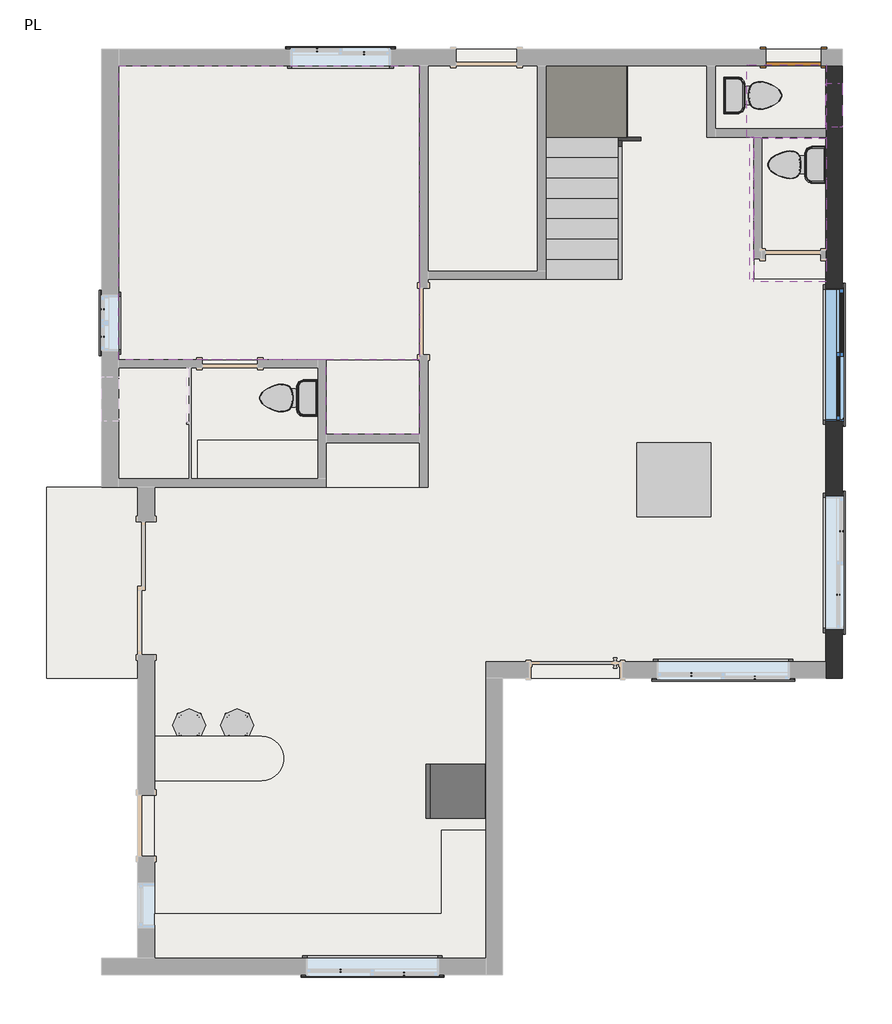
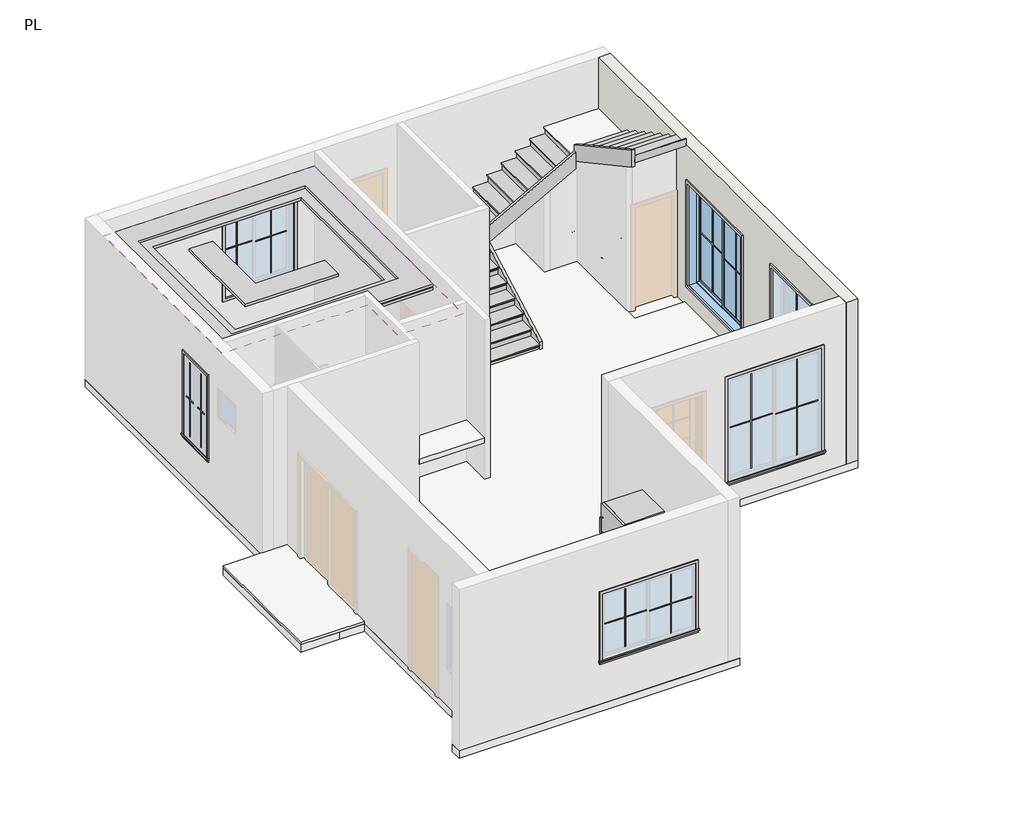
# One storey, part 2 of 2: 26 proxies, 6 slabs, 3 flow terminals, 3 furniture elements, 3 members, 3 stair flights, 2 windows, 1 covering, 2 other elements.
"""IFC4 building model written with IfcOpenShell, lengths in millimetres."""

from ifc_helpers import new_model, si_unit, point, frame, frame_2d, origin, origin_with_axes, place, context, project, spatial, polyline, circle_curve, trimmed, segment, composite_curve, outline, extrude, faceted_brep, transform, mapped, element, save
from components import proxy_1d9d56c6, generic_models_3_generic_models_3_e47a0867, muntin_pattern_2x2_muntin_pattern_2x2_bf2b9acc, muntin_pattern_2x2_muntin_pattern_2x2_111b6719, muntin_pattern_2x2_muntin_pattern_2x2_1c12c043, muntin_pattern_2x2_muntin_pattern_2x2_88561ff7, muntin_pattern_2x2_muntin_pattern_2x2_4a783bbe, trim_window_exterior_flat_with_sill_384ab7b4, trim_window_exterior_flat_with_sill_f3cea81b, trim_window_exterior_flat_with_sill_8633aa7b, trim_window_exterior_flat_with_sill_3212bfb3, trim_window_interior_flat_picture_frame_e62f86b4, trim_window_interior_flat_picture_frame_717249e1, trim_window_interior_flat_picture_frame_129e3d92, trim_window_interior_flat_picture_frame_f1d52788, door_5e1232af, toilet_domestic_3d_toilet_domestic_3d_ba6479b0, toilet_domestic_3d_toilet_domestic_3d_30431060, furniture_d95c0d1d, furniture_7b9c1204, non_monolithic_landing_3e227109, non_monolithic_landing_135483eb, stair_flight_79429955, stair_flight_d80cec9a, stair_flight_d83de971, window_80340324, window_sliding_double_6_x7_726fea71

model = new_model("IFC4")

# Units and contexts
model_context = context("Model", 3, world=origin())
ifc_project = project(units=[si_unit("LENGTHUNIT", "METRE", prefix="MILLI")], contexts=[model_context])

# Site, building, storey
site = spatial("IfcSite", under=ifc_project)
building = spatial("IfcBuilding", under=site)
storey = spatial("IfcBuildingStorey", under=building, Name="PL", Elevation=0.0)

# Proxies
placement = place(None, origin())
proxy_shape = proxy_1d9d56c6(model_context)
element("IfcBuildingElementProxy", 1, Name="Freezer-Upright : 30\" x 32\" RH", ObjectType="Freezer-Upright : 30\" x 32\" RH", at=placement, inside=storey, context=model_context, shape_type="MappedRepresentation", body=[
    mapped(proxy_shape, transform((-9045.414349, 2199.6106602, 50.8), x_axis=(0.0, 1.0, 0.0), y_axis=(-1.0, 0.0, 0.0), z_axis=(0.0, 0.0, 1.0))),
])
generic_models_3_generic_models_3_shape = generic_models_3_generic_models_3_e47a0867(model_context)
element("IfcBuildingElementProxy", 2, Name="Generic Models 3 : Generic Models 3", ObjectType="Generic Models 3 : Generic Models 3", at=placement, inside=storey, context=model_context, shape_type="MappedRepresentation", body=[
    mapped(generic_models_3_generic_models_3_shape, transform((0.0, 0.0, 0.0), x_axis=(1.0, 0.0, 0.0), y_axis=(0.0, 1.0, 0.0), z_axis=(0.0, 0.0, 1.0))),
])
muntin_pattern_2x2_muntin_pattern_2x2_shape = muntin_pattern_2x2_muntin_pattern_2x2_bf2b9acc(model_context)
element("IfcBuildingElementProxy", 3, Name="Muntin Pattern_2x2 : Muntin Pattern_2x2", ObjectType="Muntin Pattern_2x2 : Muntin Pattern_2x2", at=placement, inside=storey, context=model_context, shape_type="MappedRepresentation", body=[
    mapped(muntin_pattern_2x2_muntin_pattern_2x2_shape, transform((-3792.8752526, 4904.2502283, 539.75), x_axis=(0.0, -1.0, 0.0), y_axis=(1.0, 0.0, 0.0), z_axis=(0.0, 0.0, 1.0))),
])
element("IfcBuildingElementProxy", 4, Name="Muntin Pattern_2x2 : Muntin Pattern_2x2", ObjectType="Muntin Pattern_2x2 : Muntin Pattern_2x2", at=placement, inside=storey, context=model_context, shape_type="MappedRepresentation", body=[
    mapped(muntin_pattern_2x2_muntin_pattern_2x2_shape, transform((-3748.4252526, 5777.3752283, 539.75), x_axis=(0.0, -1.0, 0.0), y_axis=(1.0, 0.0, 0.0), z_axis=(0.0, 0.0, 1.0))),
])
element("IfcBuildingElementProxy", 5, Name="Muntin Pattern_2x2 : Muntin Pattern_2x2", ObjectType="Muntin Pattern_2x2 : Muntin Pattern_2x2", at=placement, inside=storey, context=model_context, shape_type="MappedRepresentation", body=[
    mapped(muntin_pattern_2x2_muntin_pattern_2x2_shape, transform((-3792.8752526, 7768.1003362, 539.75), x_axis=(0.0, -1.0, 0.0), y_axis=(1.0, 0.0, 0.0), z_axis=(0.0, 0.0, 1.0))),
])
element("IfcBuildingElementProxy", 6, Name="Muntin Pattern_2x2 : Muntin Pattern_2x2", ObjectType="Muntin Pattern_2x2 : Muntin Pattern_2x2", at=placement, inside=storey, context=model_context, shape_type="MappedRepresentation", body=[
    mapped(muntin_pattern_2x2_muntin_pattern_2x2_shape, transform((-3748.4252526, 8641.2253362, 539.75), x_axis=(0.0, -1.0, 0.0), y_axis=(1.0, 0.0, 0.0), z_axis=(0.0, 0.0, 1.0))),
])
element("IfcBuildingElementProxy", 7, Name="Muntin Pattern_2x2 : Muntin Pattern_2x2", ObjectType="Muntin Pattern_2x2 : Muntin Pattern_2x2", at=placement, inside=storey, context=model_context, shape_type="MappedRepresentation", body=[
    mapped(muntin_pattern_2x2_muntin_pattern_2x2_shape, transform((-5813.7627526, 3807.2877283, 539.75), x_axis=(-1.0, 0.0, 0.0), y_axis=(0.0, -1.0, 0.0), z_axis=(0.0, 0.0, 1.0))),
])
element("IfcBuildingElementProxy", 8, Name="Muntin Pattern_2x2 : Muntin Pattern_2x2", ObjectType="Muntin Pattern_2x2 : Muntin Pattern_2x2", at=placement, inside=storey, context=model_context, shape_type="MappedRepresentation", body=[
    mapped(muntin_pattern_2x2_muntin_pattern_2x2_shape, transform((-4940.6377526, 3762.8377283, 539.75), x_axis=(-1.0, 0.0, 0.0), y_axis=(0.0, -1.0, 0.0), z_axis=(0.0, 0.0, 1.0))),
])
muntin_pattern_2x2_muntin_pattern_2x2_2_shape = muntin_pattern_2x2_muntin_pattern_2x2_111b6719(model_context)
element("IfcBuildingElementProxy", 9, Name="Muntin Pattern_2x2 : Muntin Pattern_2x2", ObjectType="Muntin Pattern_2x2 : Muntin Pattern_2x2", at=placement, inside=storey, context=model_context, shape_type="MappedRepresentation", body=[
    mapped(muntin_pattern_2x2_muntin_pattern_2x2_2_shape, transform((-10319.0877526, 12348.0378362, 996.95), x_axis=(1.0, 0.0, 0.0), y_axis=(0.0, 1.0, 0.0), z_axis=(0.0, 0.0, 1.0))),
])
element("IfcBuildingElementProxy", 10, Name="Muntin Pattern_2x2 : Muntin Pattern_2x2", ObjectType="Muntin Pattern_2x2 : Muntin Pattern_2x2", at=placement, inside=storey, context=model_context, shape_type="MappedRepresentation", body=[
    mapped(muntin_pattern_2x2_muntin_pattern_2x2_2_shape, transform((-10963.6127526, 12392.4878362, 996.95), x_axis=(1.0, 0.0, 0.0), y_axis=(0.0, 1.0, 0.0), z_axis=(0.0, 0.0, 1.0))),
])
muntin_pattern_2x2_muntin_pattern_2x2_3_shape = muntin_pattern_2x2_muntin_pattern_2x2_1c12c043(model_context)
element("IfcBuildingElementProxy", 11, Name="Muntin Pattern_2x2 : Muntin Pattern_2x2", ObjectType="Muntin Pattern_2x2 : Muntin Pattern_2x2", at=placement, inside=storey, context=model_context, shape_type="MappedRepresentation", body=[
    mapped(muntin_pattern_2x2_muntin_pattern_2x2_3_shape, transform((-13914.7752526, 8447.5503362, 984.25), x_axis=(0.0, 1.0, 0.0), y_axis=(-1.0, 0.0, 0.0), z_axis=(0.0, 0.0, 1.0))),
])
muntin_pattern_2x2_muntin_pattern_2x2_4_shape = muntin_pattern_2x2_muntin_pattern_2x2_88561ff7(model_context)
element("IfcBuildingElementProxy", 12, Name="Muntin Pattern_2x2 : Muntin Pattern_2x2", ObjectType="Muntin Pattern_2x2 : Muntin Pattern_2x2", at=placement, inside=storey, context=model_context, shape_type="MappedRepresentation", body=[
    mapped(muntin_pattern_2x2_muntin_pattern_2x2_4_shape, transform((-13914.7752526, 8825.3753362, 984.25), x_axis=(0.0, -1.0, 0.0), y_axis=(1.0, 0.0, 0.0), z_axis=(0.0, 0.0, 1.0))),
])
muntin_pattern_2x2_muntin_pattern_2x2_5_shape = muntin_pattern_2x2_muntin_pattern_2x2_4a783bbe(model_context)
element("IfcBuildingElementProxy", 13, Name="Muntin Pattern_2x2 : Muntin Pattern_2x2", ObjectType="Muntin Pattern_2x2 : Muntin Pattern_2x2", at=placement, inside=storey, context=model_context, shape_type="MappedRepresentation", body=[
    mapped(muntin_pattern_2x2_muntin_pattern_2x2_5_shape, transform((-10639.7627526, -267.0309138, 996.95), x_axis=(-1.0, 0.0, 0.0), y_axis=(0.0, -1.0, 0.0), z_axis=(0.0, 0.0, 1.0))),
])
element("IfcBuildingElementProxy", 14, Name="Muntin Pattern_2x2 : Muntin Pattern_2x2", ObjectType="Muntin Pattern_2x2 : Muntin Pattern_2x2", at=placement, inside=storey, context=model_context, shape_type="MappedRepresentation", body=[
    mapped(muntin_pattern_2x2_muntin_pattern_2x2_5_shape, transform((-9766.6377526, -311.4809138, 996.95), x_axis=(-1.0, 0.0, 0.0), y_axis=(0.0, -1.0, 0.0), z_axis=(0.0, 0.0, 1.0))),
])
trim_window_exterior_flat_with_sill_shape = trim_window_exterior_flat_with_sill_384ab7b4(model_context)
element("IfcBuildingElementProxy", 15, Name="Trim-Window-Exterior-Flat : with Sill", ObjectType="Trim-Window-Exterior-Flat : with Sill", at=placement, inside=storey, context=model_context, shape_type="MappedRepresentation", body=[
    mapped(trim_window_exterior_flat_with_sill_shape, transform((-3738.9002526, 5340.8127283, 2590.8), x_axis=(0.0, 1.0, 0.0), y_axis=(0.0, 0.0, 1.0), z_axis=(1.0, 0.0, 0.0))),
])
element("IfcBuildingElementProxy", 16, Name="Trim-Window-Exterior-Flat : with Sill", ObjectType="Trim-Window-Exterior-Flat : with Sill", at=placement, inside=storey, context=model_context, shape_type="MappedRepresentation", body=[
    mapped(trim_window_exterior_flat_with_sill_shape, transform((-3738.9002526, 8204.6628362, 2590.8), x_axis=(0.0, 1.0, 0.0), y_axis=(0.0, 0.0, 1.0), z_axis=(1.0, 0.0, 0.0))),
])
element("IfcBuildingElementProxy", 17, Name="Trim-Window-Exterior-Flat : with Sill", ObjectType="Trim-Window-Exterior-Flat : with Sill", at=placement, inside=storey, context=model_context, shape_type="MappedRepresentation", body=[
    mapped(trim_window_exterior_flat_with_sill_shape, transform((-5377.2002526, 3753.3127283, 2590.8), x_axis=(1.0, 0.0, 0.0), y_axis=(0.0, 0.0, 1.0), z_axis=(0.0, -1.0, 0.0))),
])
trim_window_exterior_flat_with_sill_2_shape = trim_window_exterior_flat_with_sill_f3cea81b(model_context)
element("IfcBuildingElementProxy", 18, Name="Trim-Window-Exterior-Flat : with Sill", ObjectType="Trim-Window-Exterior-Flat : with Sill", at=placement, inside=storey, context=model_context, shape_type="MappedRepresentation", body=[
    mapped(trim_window_exterior_flat_with_sill_2_shape, transform((-10641.3502526, 12402.0128362, 2590.8), x_axis=(-1.0, 0.0, 0.0), y_axis=(0.0, 0.0, 1.0), z_axis=(0.0, 1.0, 0.0))),
])
trim_window_exterior_flat_with_sill_3_shape = trim_window_exterior_flat_with_sill_8633aa7b(model_context)
element("IfcBuildingElementProxy", 19, Name="Trim-Window-Exterior-Flat : with Sill", ObjectType="Trim-Window-Exterior-Flat : with Sill", at=placement, inside=storey, context=model_context, shape_type="MappedRepresentation", body=[
    mapped(trim_window_exterior_flat_with_sill_3_shape, transform((-13924.3002526, 8636.4628362, 2590.8), x_axis=(0.0, -1.0, 0.0), y_axis=(0.0, 0.0, 1.0), z_axis=(-1.0, 0.0, 0.0))),
])
trim_window_exterior_flat_with_sill_4_shape = trim_window_exterior_flat_with_sill_3212bfb3(model_context)
element("IfcBuildingElementProxy", 20, Name="Trim-Window-Exterior-Flat : with Sill", ObjectType="Trim-Window-Exterior-Flat : with Sill", at=placement, inside=storey, context=model_context, shape_type="MappedRepresentation", body=[
    mapped(trim_window_exterior_flat_with_sill_4_shape, transform((-10203.2002526, -321.0059138, 2286.0), x_axis=(1.0, 0.0, 0.0), y_axis=(0.0, 0.0, 1.0), z_axis=(0.0, -1.0, 0.0))),
])
trim_window_interior_flat_picture_frame_shape = trim_window_interior_flat_picture_frame_e62f86b4(model_context)
element("IfcBuildingElementProxy", 21, Name="Trim-Window-Interior-Flat : Picture Frame", ObjectType="Trim-Window-Interior-Flat : Picture Frame", at=placement, inside=storey, context=model_context, shape_type="MappedRepresentation", body=[
    mapped(trim_window_interior_flat_picture_frame_shape, transform((-3967.5002526, 5340.8127283, 2590.8), x_axis=(0.0, -1.0, 0.0), y_axis=(0.0, 0.0, 1.0), z_axis=(-1.0, 0.0, 0.0))),
])
element("IfcBuildingElementProxy", 22, Name="Trim-Window-Interior-Flat : Picture Frame", ObjectType="Trim-Window-Interior-Flat : Picture Frame", at=placement, inside=storey, context=model_context, shape_type="MappedRepresentation", body=[
    mapped(trim_window_interior_flat_picture_frame_shape, transform((-3967.5002526, 8204.6628362, 2590.8), x_axis=(0.0, -1.0, 0.0), y_axis=(0.0, 0.0, 1.0), z_axis=(-1.0, 0.0, 0.0))),
])
element("IfcBuildingElementProxy", 23, Name="Trim-Window-Interior-Flat : Picture Frame", ObjectType="Trim-Window-Interior-Flat : Picture Frame", at=placement, inside=storey, context=model_context, shape_type="MappedRepresentation", body=[
    mapped(trim_window_interior_flat_picture_frame_shape, transform((-5377.2002526, 3981.9127283, 2590.8), x_axis=(-1.0, 0.0, 0.0), y_axis=(0.0, 0.0, 1.0), z_axis=(0.0, 1.0, 0.0))),
])
trim_window_interior_flat_picture_frame_2_shape = trim_window_interior_flat_picture_frame_717249e1(model_context)
element("IfcBuildingElementProxy", 24, Name="Trim-Window-Interior-Flat : Picture Frame", ObjectType="Trim-Window-Interior-Flat : Picture Frame", at=placement, inside=storey, context=model_context, shape_type="MappedRepresentation", body=[
    mapped(trim_window_interior_flat_picture_frame_2_shape, transform((-10641.3502526, 12173.4128362, 2590.8), x_axis=(1.0, 0.0, 0.0), y_axis=(0.0, 0.0, 1.0), z_axis=(0.0, -1.0, 0.0))),
])
trim_window_interior_flat_picture_frame_3_shape = trim_window_interior_flat_picture_frame_129e3d92(model_context)
element("IfcBuildingElementProxy", 25, Name="Trim-Window-Interior-Flat : Picture Frame", ObjectType="Trim-Window-Interior-Flat : Picture Frame", at=placement, inside=storey, context=model_context, shape_type="MappedRepresentation", body=[
    mapped(trim_window_interior_flat_picture_frame_3_shape, transform((-13695.7002526, 8636.4628362, 2590.8), x_axis=(0.0, 1.0, 0.0), y_axis=(0.0, 0.0, 1.0), z_axis=(1.0, 0.0, 0.0))),
])
trim_window_interior_flat_picture_frame_4_shape = trim_window_interior_flat_picture_frame_f1d52788(model_context)
element("IfcBuildingElementProxy", 26, Name="Trim-Window-Interior-Flat : Picture Frame", ObjectType="Trim-Window-Interior-Flat : Picture Frame", at=placement, inside=storey, context=model_context, shape_type="MappedRepresentation", body=[
    mapped(trim_window_interior_flat_picture_frame_4_shape, transform((-10203.2002526, -92.4059138, 2286.0), x_axis=(-1.0, 0.0, 0.0), y_axis=(0.0, 0.0, 1.0), z_axis=(0.0, 1.0, 0.0))),
])

# Covering
element("IfcCovering", 27, ObjectType="GWB on Mtl. Stud", at=placement, inside=storey, context=model_context, shape_type="SweptSolid", body=[
    extrude(outline(polyline([(-13695.7002526, 8134.8128362), (-13695.7002526, 12173.4128362), (-9555.5002526, 12173.4128362), (-9555.5002526, 7106.1128362), (-10838.2002526, 7106.1128362), (-10838.2002526, 8134.8128362), (-13695.7002526, 8134.8128362)])), frame((0.0, 0.0, 3048.0), z_axis=(0.0, 0.0, 1.0), x_axis=(1.0, 0.0, 0.0)), (0.0, 0.0, 1.0), 107.95),
])

# Door
door_shape = door_5e1232af(model_context)
element("IfcDoor", 28, ObjectType="Single-Flush : 30\" x 84\"", at=placement, inside=storey, context=model_context, shape_type="MappedRepresentation", body=[
    mapped(door_shape, transform((-4412.0002526, 12287.7128362, 0.0), x_axis=(1.0, 0.0, 0.0), y_axis=(0.0, 1.0, 0.0), z_axis=(0.0, 0.0, 1.0))),
])

# Flow terminals
toilet_domestic_3d_toilet_domestic_3d_shape = toilet_domestic_3d_toilet_domestic_3d_ba6479b0(model_context)
toilet_domestic_3d_toilet_domestic_3d_2_shape = toilet_domestic_3d_toilet_domestic_3d_30431060(model_context)
element("IfcFlowTerminal", 29, ObjectType="Toilet-Domestic-3D : Toilet-Domestic-3D", at=placement, inside=storey, context=model_context, shape_type="MappedRepresentation", body=[
    mapped(toilet_domestic_3d_toilet_domestic_3d_shape, transform((-11447.1962799, 7607.7628362, 0.0), x_axis=(0.0, -1.0, 0.0), y_axis=(1.0, 0.0, 0.0), z_axis=(0.0, 0.0, 1.0))),
    mapped(toilet_domestic_3d_toilet_domestic_3d_2_shape, transform((-11447.1962799, 7607.7628362, 0.0), x_axis=(0.0, -1.0, 0.0), y_axis=(1.0, 0.0, 0.0), z_axis=(0.0, 0.0, 1.0))),
])
element("IfcFlowTerminal", 30, ObjectType="Toilet-Domestic-3D : Toilet-Domestic-3D", at=placement, inside=storey, context=model_context, shape_type="MappedRepresentation", body=[
    mapped(toilet_domestic_3d_toilet_domestic_3d_shape, transform((-4459.6252526, 10814.5128362, 0.0), x_axis=(0.0, -1.0, 0.0), y_axis=(1.0, 0.0, 0.0), z_axis=(0.0, 0.0, 1.0))),
    mapped(toilet_domestic_3d_toilet_domestic_3d_2_shape, transform((-4459.6252526, 10814.5128362, 0.0), x_axis=(0.0, -1.0, 0.0), y_axis=(1.0, 0.0, 0.0), z_axis=(0.0, 0.0, 1.0))),
])
element("IfcFlowTerminal", 31, ObjectType="Toilet-Domestic-3D : Toilet-Domestic-3D", at=placement, inside=storey, context=model_context, shape_type="MappedRepresentation", body=[
    mapped(toilet_domestic_3d_toilet_domestic_3d_shape, transform((-4876.9108447, 11767.1178103, 0.0), x_axis=(0.0, 1.0, 0.0), y_axis=(-1.0, 0.0, 0.0), z_axis=(0.0, 0.0, 1.0))),
    mapped(toilet_domestic_3d_toilet_domestic_3d_2_shape, transform((-4876.9108447, 11767.1178103, 0.0), x_axis=(0.0, 1.0, 0.0), y_axis=(-1.0, 0.0, 0.0), z_axis=(0.0, 0.0, 1.0))),
])

# Furniture
furniture_shape = furniture_d95c0d1d(model_context)
element("IfcFurniture", 32, at=placement, inside=storey, context=model_context, shape_type="MappedRepresentation", body=[
    mapped(furniture_shape, transform((-12063.7502526, 3107.9940862, 0.0), x_axis=(1.0, 0.0, 0.0), y_axis=(0.0, 1.0, 0.0), z_axis=(0.0, 0.0, 1.0))),
])
element("IfcFurniture", 33, at=placement, inside=storey, context=model_context, shape_type="MappedRepresentation", body=[
    mapped(furniture_shape, transform((-12724.1502526, 3107.9940862, 0.0), x_axis=(1.0, 0.0, 0.0), y_axis=(0.0, 1.0, 0.0), z_axis=(0.0, 0.0, 1.0))),
])
furniture_2_shape = furniture_7b9c1204(model_context)
element("IfcFurniture", 34, ObjectType="40\" x 40\"", at=placement, inside=storey, context=model_context, shape_type="MappedRepresentation", body=[
    mapped(furniture_2_shape, transform((-6000.2228839, 6543.7734919, 50.8), x_axis=(1.0, 0.0, 0.0), y_axis=(0.0, 1.0, 0.0), z_axis=(0.0, 0.0, 1.0))),
])

# Members
element("IfcMember", 35, ObjectType="Stringer - 2\" Width", at=placement, inside=storey, context=model_context, shape_type="SweptSolid", body=[
    extrude(outline(polyline([(9239.7128362, 0.0), (9239.7128362, 206.7436667), (11144.7128362, 1245.8345758), (11144.7128362, 898.6406619), (9497.2049561, 0.0), (9239.7128362, 0.0)])), frame((-6818.6502526, 0.0, 0.0), z_axis=(1.0, 0.0, 0.0), x_axis=(0.0, 1.0, 0.0)), (0.0, 0.0, 1.0), 50.8),
])
element("IfcMember", 36, ObjectType="Stringer - 2\" Width", at=placement, inside=storey, context=model_context, shape_type="SweptSolid", body=[
    extrude(outline(polyline([(1377.4527576, -6818.6502526), (1030.2588436, -6818.6502526), (2017.3952072, -5008.9002526), (2364.5891212, -5008.9002526), (1377.4527576, -6818.6502526)])), frame((0.0, 11144.7128362, 0.0), z_axis=(0.0, 1.0, 0.0), x_axis=(0.0, 0.0, 1.0)), (0.0, 0.0, 1.0), 50.8),
])
element("IfcMember", 37, ObjectType="Stringer - 2\" Width", at=placement, inside=storey, context=model_context, shape_type="SweptSolid", body=[
    extrude(outline(polyline([(11195.5128362, 2492.7436667), (11195.5128362, 2145.5497528), (9239.7128362, 3212.3497528), (9239.7128362, 3559.5436667), (11195.5128362, 2492.7436667)])), frame((-5008.9002526, 0.0, 0.0), z_axis=(1.0, 0.0, 0.0), x_axis=(0.0, 1.0, 0.0)), (0.0, 0.0, 1.0), 50.8),
])

# Slabs
element("IfcSlab", 38, ObjectType="4\"", at=placement, inside=storey, context=model_context, shape_type="SweptSolid", body=[
    extrude(outline(polyline([(-9555.5002526, 6991.8128362), (-9555.5002526, 6382.2128362), (-10838.2002526, 6382.2128362), (-10838.2002526, 6991.8128362), (-9555.5002526, 6991.8128362)])), frame((0.0, 0.0, 812.8), z_axis=(0.0, 0.0, 1.0), x_axis=(1.0, 0.0, 0.0)), (0.0, 0.0, 1.0), 101.6),
    extrude(outline(polyline([(-10952.5002526, 7029.9128362), (-10952.5002526, 6496.5128362), (-12604.2306335, 6496.5128362), (-12604.2306335, 7029.9128362), (-10952.5002526, 7029.9128362)])), frame((0.0, 0.0, 812.8), z_axis=(0.0, 0.0, 1.0), x_axis=(1.0, 0.0, 0.0)), (0.0, 0.0, 1.0), 101.6),
    extrude(outline(polyline([(-9250.7002526, 517.1940862), (-9250.7002526, 1664.5013456), (-8641.1002526, 1664.5013456), (-8641.1002526, -92.4059138), (-13200.4002526, -92.4059138), (-13200.4002526, 517.1940862), (-9250.7002526, 517.1940862)])), frame((0.0, 0.0, 812.8), z_axis=(0.0, 0.0, 1.0), x_axis=(1.0, 0.0, 0.0)), (0.0, 0.0, 1.0), 101.6),
])
element("IfcSlab", 39, ObjectType="4\"", at=placement, inside=storey, context=model_context, shape_type="SweptSolid", body=[
    extrude(outline(composite_curve([segment(trimmed(circle_curve(frame_2d((-11727.2002526, 2650.7940862)), 304.8), [point((-11727.2002526, 2955.5940862))], [point((-11727.2002526, 2345.9940862))], False, "CARTESIAN"), True, "CONTINUOUS"), segment(polyline([(-11727.2002526, 2345.9940862), (-13200.4002526, 2345.9940862), (-13200.4002526, 2955.5940862), (-11727.2002526, 2955.5940862)]), True, "CONTINUOUS")], self_intersect=False)), frame((0.0, 0.0, 863.6), z_axis=(0.0, 0.0, 1.0), x_axis=(1.0, 0.0, 0.0)), (0.0, 0.0, 1.0), 101.6),
])
element("IfcSlab", 40, ObjectType="6\"", at=placement, inside=storey, context=model_context, shape_type="SweptSolid", body=[
    extrude(outline(polyline([(-3738.9002526, 12402.0128362), (-3738.9002526, 3753.3127283), (-8412.5002526, 3753.3127283), (-8412.5002526, -321.0059138), (-13924.3002526, -321.0059138), (-13924.3002526, -92.4059138), (-13429.0002526, -92.4059138), (-13429.0002526, 3752.3673766), (-13924.3002526, 3752.3673766), (-14686.3002526, 3752.3673766), (-14686.3002526, 6382.2128362), (-13924.3002526, 6382.2128362), (-13924.3002526, 12402.0128362), (-3738.9002526, 12402.0128362)])), frame((0.0, 0.0, -152.4), z_axis=(0.0, 0.0, 1.0), x_axis=(1.0, 0.0, 0.0)), (0.0, 0.0, 1.0), 152.4),
])
element("IfcSlab", 41, ObjectType="HALL FLOORING", at=placement, inside=storey, context=model_context, shape_type="SweptSolid", body=[
    extrude(outline(polyline([(-7815.6002526, 9239.7128362), (-7815.6002526, 12173.4128362), (-5599.4131221, 12173.4128362), (-5599.4131221, 11195.5128362), (-4958.1002526, 11195.5128362), (-4958.1002526, 9239.7128362), (-3967.5002526, 9239.7128362), (-3967.5002526, 3981.9127283), (-6774.2002526, 3981.9127283), (-6774.2002526, 3753.3127283), (-8044.2002526, 3753.3127283), (-8044.2002526, 3981.9127283), (-8641.1002526, 3981.9127283), (-8641.1002526, -92.4059138), (-13200.4002526, -92.4059138), (-13200.4002526, 4077.1628362), (-13429.0002526, 4077.1628362), (-13429.0002526, 3752.3673766), (-14686.3002526, 3752.3673766), (-14686.3002526, 6382.2128362), (-13429.0002526, 6382.2128362), (-13429.0002526, 5905.9628362), (-13200.4002526, 5905.9628362), (-13200.4002526, 6382.2128362), (-10838.2002526, 6382.2128362), (-10838.2002526, 6991.8128362), (-9555.5002526, 6991.8128362), (-9555.5002526, 6382.2128362), (-9441.2002526, 6382.2128362), (-9441.2002526, 8134.8128362), (-13695.7002526, 8134.8128362), (-13695.7002526, 12173.4128362), (-9441.2002526, 12173.4128362), (-9441.2002526, 9239.7128362), (-7815.6002526, 9239.7128362)])), origin_with_axes(), (0.0, 0.0, 1.0), 50.8),
])
non_monolithic_landing_shape = non_monolithic_landing_3e227109(model_context)
element("IfcSlab", 42, ObjectType="Non-Monolithic Landing", at=placement, inside=storey, context=model_context, shape_type="MappedRepresentation", body=[
    mapped(non_monolithic_landing_shape, transform((0.0, 0.0, 0.0), x_axis=(1.0, 0.0, 0.0), y_axis=(0.0, 1.0, 0.0), z_axis=(0.0, 0.0, 1.0))),
])
non_monolithic_landing_2_shape = non_monolithic_landing_135483eb(model_context)
element("IfcSlab", 43, ObjectType="Non-Monolithic Landing", at=placement, inside=storey, context=model_context, shape_type="MappedRepresentation", body=[
    mapped(non_monolithic_landing_2_shape, transform((0.0, 0.0, 0.0), x_axis=(1.0, 0.0, 0.0), y_axis=(0.0, 1.0, 0.0), z_axis=(0.0, 0.0, 1.0))),
])

# Stair flights
stair_flight_shape = stair_flight_79429955(model_context)
element("IfcStairFlight", 44, ObjectType="2\" Tread 1\" Nosing 1/4\" Riser", at=placement, inside=storey, context=model_context, shape_type="MappedRepresentation", body=[
    mapped(stair_flight_shape, transform((0.0, 0.0, 0.0), x_axis=(1.0, 0.0, 0.0), y_axis=(0.0, 1.0, 0.0), z_axis=(0.0, 0.0, 1.0))),
])
stair_flight_2_shape = stair_flight_d80cec9a(model_context)
element("IfcStairFlight", 45, ObjectType="2\" Tread 1\" Nosing 1/4\" Riser", at=placement, inside=storey, context=model_context, shape_type="MappedRepresentation", body=[
    mapped(stair_flight_2_shape, transform((0.0, 0.0, 0.0), x_axis=(1.0, 0.0, 0.0), y_axis=(0.0, 1.0, 0.0), z_axis=(0.0, 0.0, 1.0))),
])
stair_flight_3_shape = stair_flight_d83de971(model_context)
element("IfcStairFlight", 46, ObjectType="2\" Tread 1\" Nosing 1/4\" Riser", at=placement, inside=storey, context=model_context, shape_type="MappedRepresentation", body=[
    mapped(stair_flight_3_shape, transform((0.0, 0.0, 0.0), x_axis=(1.0, 0.0, 0.0), y_axis=(0.0, 1.0, 0.0), z_axis=(0.0, 0.0, 1.0))),
])

# Wall
element("IfcWall", 47, ObjectType="10\"", at=placement, inside=storey, context=model_context, shape_type="Brep", body=[
    faceted_brep([(-3967.5002526, 12173.4128362, 0.0), (-3967.5002526, 11309.8128362, 0.0), (-3967.5002526, 11195.5128362, 0.0), (-3967.5002526, 9633.4128362, 0.0), (-3967.5002526, 9519.1128362, 0.0), (-3967.5002526, 3981.9127283, 0.0), (-3967.5002526, 3753.3127283, 0.0), (-3967.5002526, 3753.3127283, 3352.8), (-3967.5002526, 3981.9127283, 3352.8), (-3967.5002526, 12173.4128362, 3352.8), (-3967.5002526, 4426.4127283, 2590.8), (-3967.5002526, 4426.4127283, 457.2), (-3967.5002526, 6255.2127283, 457.2), (-3967.5002526, 6255.2127283, 2590.8), (-3967.5002526, 7290.2628362, 2590.8), (-3967.5002526, 7290.2628362, 457.2), (-3967.5002526, 9119.0628362, 457.2), (-3967.5002526, 9119.0628362, 2590.8), (-3967.5002526, 11328.8628362, 2133.6), (-3967.5002526, 11328.8628362, 1524.0), (-3967.5002526, 11938.4628362, 1524.0), (-3967.5002526, 11938.4628362, 2133.6), (-3738.9002526, 12173.4128362, 0.0), (-3738.9002526, 12173.4128362, 3352.8), (-3738.9002526, 3753.3127283, 3352.8), (-3738.9002526, 3753.3127283, 0.0), (-3738.9002526, 4426.4127283, 2590.8), (-3738.9002526, 6255.2127283, 2590.8), (-3738.9002526, 6255.2127283, 457.2), (-3738.9002526, 4426.4127283, 457.2), (-3738.9002526, 7290.2628362, 2590.8), (-3738.9002526, 9119.0628362, 2590.8), (-3738.9002526, 9119.0628362, 457.2), (-3738.9002526, 7290.2628362, 457.2), (-3738.9002526, 11328.8628362, 2133.6), (-3738.9002526, 11938.4628362, 2133.6), (-3738.9002526, 11938.4628362, 1524.0), (-3738.9002526, 11328.8628362, 1524.0)], [[[0, 1, 2, 3, 4, 5, 6, 7, 8, 9], [10, 11, 12, 13], [14, 15, 16, 17], [18, 19, 20, 21]], [[22, 23, 24, 25], [26, 27, 28, 29], [30, 31, 32, 33], [34, 35, 36, 37]], [[6, 5, 4, 3, 2, 1, 0, 22, 25]], [[9, 8, 7, 24, 23]], [[0, 9, 23, 22]], [[7, 6, 25, 24]], [[11, 10, 26, 29]], [[12, 11, 29, 28]], [[13, 12, 28, 27]], [[10, 13, 27, 26]], [[15, 14, 30, 33]], [[16, 15, 33, 32]], [[17, 16, 32, 31]], [[14, 17, 31, 30]], [[19, 18, 34, 37]], [[20, 19, 37, 36]], [[21, 20, 36, 35]], [[18, 21, 35, 34]]]),
])

# Windows
window_shape = window_80340324(model_context)
element("IfcWindow", 48, ObjectType="Fixed : 24\" x 24\"", at=placement, inside=storey, context=model_context, shape_type="MappedRepresentation", body=[
    mapped(window_shape, transform((-3853.2002526, 11595.5628362, 609.6), x_axis=(0.0, -1.0, 0.0), y_axis=(1.0, 0.0, 0.0), z_axis=(0.0, 0.0, 1.0))),
])
window_sliding_double_6_x7_shape = window_sliding_double_6_x7_726fea71(model_context)
element("IfcWindow", 49, ObjectType="Window-Sliding-Double : 6'X7'", at=placement, inside=storey, context=model_context, shape_type="MappedRepresentation", body=[
    mapped(window_sliding_double_6_x7_shape, transform((-3849.3902526, 8204.6628362, -457.2), x_axis=(0.0, -1.0, 0.0), y_axis=(1.0, 0.0, 0.0), z_axis=(0.0, 0.0, 1.0))),
])

save(model, "model.ifc")

# Revit data of these elements
# Type "Freezer-Upright : 30\" x 32\" RH"
#   Assembly Code = "E1090400"
#   Depth = 2' - 7 3/4"
#   Handle = 2' - 2 1/2"
#   Height = 5' - 10"
#   Rear Clearance = 0' - 2"
#   Width = 2' - 5 3/8"
#   Material = Metal - Paint Finish - Ivory,Glossy
#   Default Elevation = 0
# Type "Muntin Pattern_2x2 : Muntin Pattern_2x2"
#   Width [instance default] = 4' - 0"
#   Thickness = 0' - 0 1/2"
#   Height [instance default] = 4' - 0"
#   Distance = 0' - 0 3/4"
#   Interior Material [instance default] = none
#   Exterior Material [instance default] = none
#   Default Elevation = 0
# Type "Trim-Window-Exterior-Flat : with Sill"
#   Trim Width = 0' - 2 1/4"
#   Trim Thickness_Picture Frame = 0' - 1 1/4"
#   Trim Thickness_with Sill = 0' - 0 3/4"
#   Sill Thickness = 0' - 1 1/4"
#   Opening Width [instance default] = 2' - 0"
#   Opening Height [instance default] = 3' - 0"
#   Default Elevation = 4' - 0"
#   Sill = yes
#   Picture Frame = no
#   Trim Material [instance default] = none
# Type "Trim-Window-Interior-Flat : Picture Frame"
#   Trim Thickness_Picture Frame = 0' - 1 1/4"
#   Trim Width = 0' - 2 1/4"
#   Trim Thickness_with Sill = 0' - 0 3/4"
#   Sill Thickness = 0' - 1 1/4"
#   Opening Width [instance default] = 2' - 0"
#   Opening Height [instance default] = 3' - 0"
#   Default Elevation = 4' - 0"
#   Sill = no
#   Picture Frame = yes
#   Trim Material [instance default] = none
# Type "GWB on Mtl. Stud"
#   Assembly Code = "C3030220"
#   built-in parameter 1002203 = 1 (stored number, unit not read)
#   built-in parameter 1002202 = 1 (stored number, unit not read)
#   Layers, outside or top first: 0' - 3 5/8" "Metal Stud Layer" (function 1); 0' - 0 5/8" "Gypsum Wall Board" (function 5)
# Type "Single-Flush : 30\" x 84\""
#   Type Mark = "4"
#   Construction Type Id = "MDOOR"
#   Assembly Code = "C1020"
#   Analytic Construction = "Metal"
#   Thickness = 0' - 2"
#   Heat Transfer Coefficient (U) = 0.651978 BTU/(h·ft²·°F)
#   Height = 7' - 0"
#   Trim Projection Ext = 0' - 1"
#   Trim Projection Int = 0' - 1"
#   Trim Width = 0' - 3"
#   Width = 2' - 6"
#   Define Thermal Properties by = 1
#   Define Thermal Properties by = 1
#   Door Material = Door - Panel
#   Frame Material = Door - Frame
#   Visual Light Transmittance = 0
#   Solar Heat Gain Coefficient = 0
#   Function = (empty or 0)
#   Wall Closure = (empty or 0)
# Type "Toilet-Domestic-3D : Toilet-Domestic-3D"
#   Assembly Code = "D2010110"
#   Toilet - Bowl/Basin Material = Porcelain, Linen
#   Toilet - Seat Material = Laminate, Linen, Matte
#   Default Elevation = 0
# Type
#   Default Elevation = 0
# Type "40\" x 40\""
#   Assembly Code = "E2020200"
#   Height = 1' - 5"
#   Length = 3' - 4"
#   Width = 3' - 4"
#   Default Elevation = 0
# Type "4\""
#   Assembly Code = "B1010"
#   Function = 0
#   Layers, outside or top first: 0' - 1" "KITCHEN BED" (function 1); 0' - 3" no material (function 1)
# Type "6\""
#   Assembly Code = "B1010"
#   Function = 0
#   Layers, outside or top first: 0' - 6" "Gypsum Wall Board" (function 1)
# Type "HALL FLOORING"
#   Assembly Code = "B1010"
#   Function = 0
#   Layers, outside or top first: 0' - 1" "HALL FLOORING" (function 1); 0' - 1" no material (function 1)
# Type "10\""
#   Assembly Code = "B2010"
#   Layers, outside or top first: 0' - 9" "Gypsum Wall Board" (function 1)
# Type "Fixed : 24\" x 24\""
#   Type Mark = "3"
#   Construction Type Id = "GSP4R"
#   Assembly Code = "B2020100"
#   Analytic Construction = "1/8 in Pilkington single glazing"
#   Visual Light Transmittance = 0.9
#   Solar Heat Gain Coefficient = 0.78
#   Heat Transfer Coefficient (U) = 0.6496 BTU/(h·ft²·°F)
#   Height = 2' - 0"
#   Default Sill Height = 3' - 0"
#   Width = 2' - 0"
#   Window Inset = 0' - 0 3/4"
#   Define Thermal Properties by = 1
#   Define Thermal Properties by = 1
#   Glass Pane Material = Glass
#   Sash Material = Sash
#   Wall Closure = (empty or 0)
# Type "Window-Sliding-Double : 6'X7'"
#   Type Mark = "19"
#   Fire Rating = "0.5h"
#   Assembly Code = "B2020100"
#   Analytic Construction = "Double glazing - domestic"
#   Window Inset [instance default] = 0' - 0"
#   Wall Thickness [instance default] = 0' - 6"
#   Visual Light Transmittance = 0.81
#   Thermal Resistance (R) = 1.8146 (h·ft²·°F)/BTU
#   Solar Heat Gain Coefficient = 0.76
#   Muntin Width = 2' - 8 5/8"
#   Muntin Height = 6' - 6 1/4"
#   Interior Wall Closure [instance default] = 0' - 2 3/4"
#   Heat Transfer Coefficient (U) = 0.5511 BTU/(h·ft²·°F)
#   Frame Extension [instance default] = 0' - 0 1/4"
#   Exterior Wall Closure [instance default] = 0' - 1 1/4"
#   Rough Width = 6' - 0 1/2"
#   Rough Height = 7' - 0 1/2"
#   Height = 7' - 0"
#   Extension Jamb [instance default] = 0' - 2 3/4"
#   Default Sill Height = 3' - 0"
#   Width = 6' - 0"
#   Interior Trim Visibility [instance default] = yes
#   Indicator Visibility [instance default] = yes
#   Exterior Trim Visibility [instance default] = yes
#   Muntin Visibility = yes
#   Extension Jamb Visibility [instance default] = yes
#   Muntin Pattern = Muntin Pattern_2x2 : Muntin Pattern_2x2
#   Interior Trim Material = Wood - Stained
#   Interior Trim = Trim-Window-Interior-Flat : Picture Frame
#   Interior Frame Material = Wood - Stained
#   Glass Panel Material = Glass
#   Exterior Trim Material = Clad - White
#   Exterior Trim = Trim-Window-Exterior-Flat : with Sill
#   Exterior Frame Material = Clad - White
#   Wall Closure = (empty or 0)
# Element 1 (IfcBuildingElementProxy, "Freezer-Upright : 30\" x 32\" RH")
#   Phase Created = New Construction
#   Materials on its faces: "Metal - Paint Finish - Ivory,Glossy", "Metal - Chrome", "Metal - Paint Finish - Black,Glossy"
# Element 2 (IfcBuildingElementProxy, "Generic Models 3 : Generic Models 3")
#   Phase Created = New Construction
#   Materials on its faces: "Wall Material (1)", "1 light"
# Elements 3, 4, 5, 6, 7, 8 (IfcBuildingElementProxy, "Muntin Pattern_2x2 : Muntin Pattern_2x2")
#   Width = 2' - 8 5/8"
#   Height = 6' - 6 1/4"
#   Interior Material = Wood - Stained
#   Exterior Material = Clad - White
#   Phase Created = New Construction
#   Materials on its faces: "Clad - White", "Wood - Stained"
# Elements 9, 10 (IfcBuildingElementProxy, "Muntin Pattern_2x2 : Muntin Pattern_2x2")
#   Width = 1' - 11 5/8"
#   Height = 5' - 0 1/4"
#   Interior Material = Wood - Stained
#   Exterior Material = Clad - White
#   Phase Created = New Construction
#   Materials on its faces: "Clad - White", "Wood - Stained"
# Elements 11, 12 (IfcBuildingElementProxy, "Muntin Pattern_2x2 : Muntin Pattern_2x2")
#   Width = 0' - 9 5/8"
#   Height = 5' - 0 1/2"
#   Interior Material = Wood - Stained
#   Exterior Material = Clad - White
#   Phase Created = New Construction
#   Materials on its faces: "Clad - White", "Wood - Stained"
# Elements 13, 14 (IfcBuildingElementProxy, "Muntin Pattern_2x2 : Muntin Pattern_2x2")
#   Width = 2' - 8 5/8"
#   Height = 4' - 0 1/4"
#   Interior Material = Wood - Stained
#   Exterior Material = Clad - White
#   Phase Created = New Construction
#   Materials on its faces: "Clad - White", "Wood - Stained"
# Elements 15, 16, 17 (IfcBuildingElementProxy, "Trim-Window-Exterior-Flat : with Sill")
#   Opening Width = 6' - 0"
#   Opening Height = 7' - 0"
#   Trim Material = Clad - White
#   Phase Created = New Construction
#   Materials on its faces: "Clad - White"
# Element 18 (IfcBuildingElementProxy, "Trim-Window-Exterior-Flat : with Sill")
#   Opening Width = 4' - 6"
#   Opening Height = 5' - 6"
#   Trim Material = Clad - White
#   Phase Created = New Construction
#   Materials on its faces: "Clad - White"
# Element 19 (IfcBuildingElementProxy, "Trim-Window-Exterior-Flat : with Sill")
#   Opening Width = 2' - 6"
#   Opening Height = 5' - 6"
#   Trim Material = Clad - White
#   Phase Created = New Construction
#   Materials on its faces: "Clad - White"
# Element 20 (IfcBuildingElementProxy, "Trim-Window-Exterior-Flat : with Sill")
#   Opening Width = 6' - 0"
#   Opening Height = 4' - 6"
#   Trim Material = Clad - White
#   Phase Created = New Construction
#   Materials on its faces: "Clad - White"
# Elements 21, 22, 23 (IfcBuildingElementProxy, "Trim-Window-Interior-Flat : Picture Frame")
#   Opening Width = 6' - 0"
#   Opening Height = 7' - 0"
#   Trim Material = Wood - Stained
#   Phase Created = New Construction
#   Materials on its faces: "Wood - Stained"
# Element 24 (IfcBuildingElementProxy, "Trim-Window-Interior-Flat : Picture Frame")
#   Opening Width = 4' - 6"
#   Opening Height = 5' - 6"
#   Trim Material = Wood - Stained
#   Phase Created = New Construction
#   Materials on its faces: "Wood - Stained"
# Element 25 (IfcBuildingElementProxy, "Trim-Window-Interior-Flat : Picture Frame")
#   Opening Width = 2' - 6"
#   Opening Height = 5' - 6"
#   Trim Material = Wood - Stained
#   Phase Created = New Construction
#   Materials on its faces: "Wood - Stained"
# Element 26 (IfcBuildingElementProxy, "Trim-Window-Interior-Flat : Picture Frame")
#   Opening Width = 6' - 0"
#   Opening Height = 4' - 6"
#   Trim Material = Wood - Stained
#   Phase Created = New Construction
#   Materials on its faces: "Wood - Stained"
# Element 27 (IfcCovering, "GWB on Mtl. Stud")
#   Height Offset From Level = 10' - 0"
#   Phase Created = New Construction
#   Materials on its faces: "Gypsum Wall Board", "Metal Stud Layer"
# Element 28 (IfcDoor, "Single-Flush : 30\" x 84\"")
#   Phase Created = New Construction
#   Materials on its faces: "Door - Frame", "Door - Panel"
# Element 29 (IfcFlowTerminal, "Toilet-Domestic-3D : Toilet-Domestic-3D")
#   Mark = "1"
#   Phase Created = New Construction
#   Materials on its faces: "Porcelain, Linen", "Laminate, Linen, Matte"
# Element 30 (IfcFlowTerminal, "Toilet-Domestic-3D : Toilet-Domestic-3D")
#   Mark = "2"
#   Phase Created = New Construction
#   Materials on its faces: "Porcelain, Linen", "Laminate, Linen, Matte"
# Element 31 (IfcFlowTerminal, "Toilet-Domestic-3D : Toilet-Domestic-3D")
#   Mark = "3"
#   Phase Created = New Construction
#   Materials on its faces: "Porcelain, Linen", "Laminate, Linen, Matte"
# Elements 32, 33 (IfcFurniture)
#   Phase Created = New Construction
#   Materials on its faces: "Metal - Chrome", "Wood - Birch"
# Element 34 (IfcFurniture, "40\" x 40\"")
#   Phase Created = New Construction
#   Materials on its faces: "Metal - Steel, Polished", "Glass - Clear, Grey"
# Elements 35, 36, 37 (IfcMember, "Stringer - 2\" Width")
#   Phase Created = New Construction
# Element 38 (IfcSlab, "4\"")
#   Height Offset From Level = 3' - 0"
#   Phase Created = New Construction
#   Materials on its faces: "Default Floor", "KITCHEN BED"
# Element 39 (IfcSlab, "4\"")
#   built-in parameter 1001955 = 3.14159 (stored number, unit not read)
#   Height Offset From Level = 3' - 2"
#   Phase Created = New Construction
#   Materials on its faces: "Default Floor", "KITCHEN BED"
# Element 40 (IfcSlab, "6\"")
#   Height Offset From Level = 0' - 0"
#   Phase Created = New Construction
#   Materials on its faces: "Gypsum Wall Board"
# Element 41 (IfcSlab, "HALL FLOORING")
#   Height Offset From Level = 0' - 2"
#   Phase Created = New Construction
#   Materials on its faces: "Default Floor", "HALL FLOORING"
# Elements 42, 43 (IfcSlab, "Non-Monolithic Landing")
#   Phase Created = New Construction
# Elements 44, 45, 46 (IfcStairFlight, "2\" Tread 1\" Nosing 1/4\" Riser")
#   Phase Created = New Construction
# Element 47 (IfcWall, "10\"")
#   Top Offset = 0' - 0"
#   Base Offset = 0' - 0"
#   Unconnected Height = 11' - 0"
#   wall height = 11' - 0"
#   Phase Created = New Construction
#   Base Constraint = PL
#   Materials on its faces: "Gypsum Wall Board"
# Element 48 (IfcWindow, "Fixed : 24\" x 24\"")
#   Mark = "4"
#   Phase Created = New Construction
#   Materials on its faces: "Sash", "Glass"
# Element 49 (IfcWindow, "Window-Sliding-Double : 6'X7'")
#   Mark = "2"
#   Window Inset = 0' - 0"
#   Interior Wall Closure = 0' - 2 3/4"
#   Frame Extension = 0' - 0 1/4"
#   Exterior Wall Closure = 0' - 1 1/4"
#   Interior Trim Visibility = yes
#   Indicator Visibility = yes
#   Exterior Trim Visibility = yes
#   Phase Created = New Construction
#   Materials on its faces: "Wood - Stained", "Glass", "Clad - White"
# Materials
#   "Metal - Paint Finish - Ivory,Glossy": colour RGB 247 247 239, transparency 0
#   "Metal Stud Layer": class "Metal", colour RGB 199 199 199, transparency 0, Description = "Light gauge steel framing, thermal air layer", Cost = 0
#   "Gypsum Wall Board": class "Generic", colour RGB 228 228 228, transparency 0, Description = "Gypsum Wall Board", Cost = 0
#   "Door - Panel": class "Wood", colour RGB 210 159 95, transparency 0, Cost = 0
#   "Door - Frame": colour RGB 118 70 51, transparency 0, Cost = 0
#   "Porcelain, Linen": class "Ceramic", colour RGB 249 239 230, transparency 0, Description = "Porcelain, linen", Cost = 0
#   "Laminate, Linen, Matte": class "Plastic", colour RGB 249 239 230, transparency 0, Description = "Plastic Laminate - Linen, Matte", Cost = 0
#   "KITCHEN BED": class "Generic", colour RGB 45 47 49, transparency 0, Cost = 0
#   "HALL FLOORING": class "Generic", colour RGB 120 120 120, transparency 0, Cost = 0
#   "Glass": class "Glass", colour RGB 0 128 192, transparency 0.75, Description = "Soda Lime Glass", Cost = 0
#   "Sash": class "Wood", colour RGB 224 178 126, transparency 0, Cost = 0
#   "Wood - Stained": class "Wood", colour RGB 224 178 126, transparency 0, Cost = 0
#   "Clad - White": class "Wood", colour RGB 242 242 238, transparency 0, Cost = 0
#   "Metal - Chrome": colour RGB 177 177 177, transparency 0
#   "Metal - Paint Finish - Black,Glossy": colour RGB 0 0 0, transparency 0
#   "Wall Material (1)": colour RGB 80 80 80, transparency 0, Cost = 0
#   "1 light": colour RGB 242 242 242, transparency 1
#   "Wood - Birch": colour RGB 210 159 95, transparency 0
#   "Metal - Steel, Polished": colour RGB 57 57 57, transparency 0
#   "Glass - Clear, Grey": colour RGB 252 255 255, transparency 0.64
#   "Default Floor": colour RGB 128 128 128, transparency 0, Cost = 0
